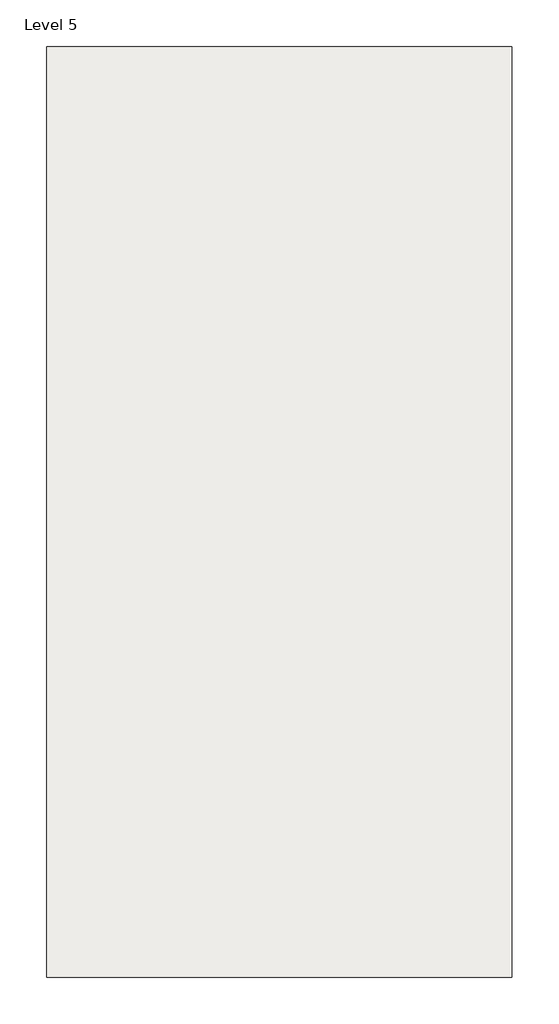
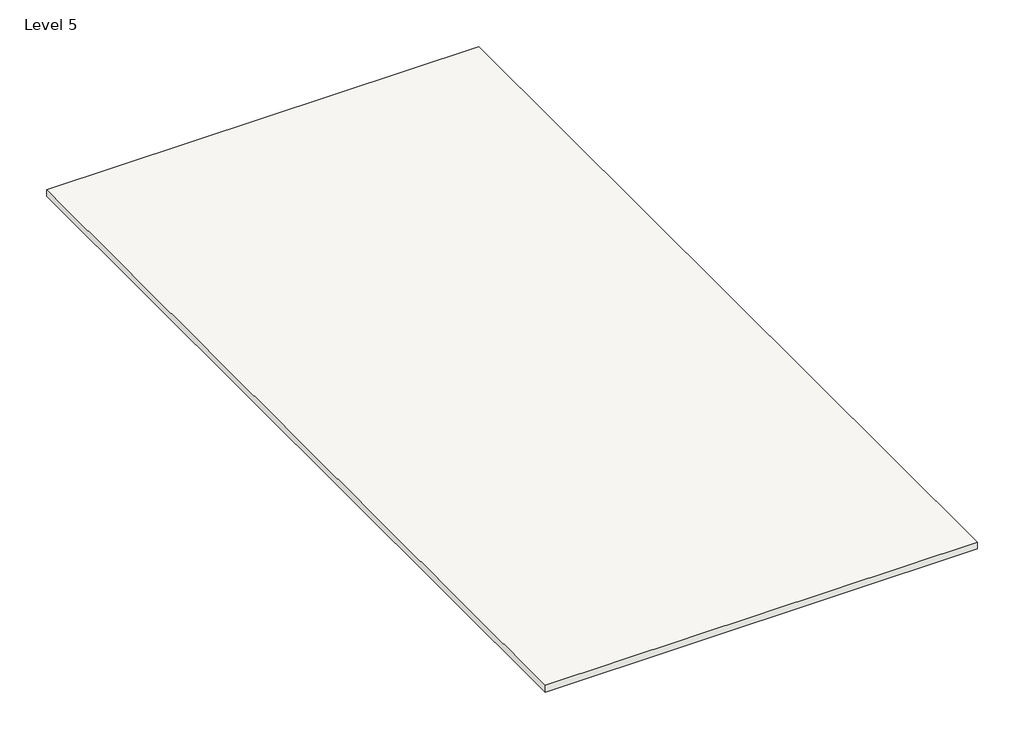
# One storey: 1 roof.
"""IFC4 building model written with IfcOpenShell, lengths in millimetres."""

from ifc_helpers import new_model, si_unit, frame, origin, place, context, project, spatial, polyline, outline, extrude, element, save

model = new_model("IFC4")

# Units and contexts
model_context = context("Model", 3, world=origin())
ifc_project = project(units=[si_unit("LENGTHUNIT", "METRE", prefix="MILLI")], contexts=[model_context])

# Site, building, storey
site = spatial("IfcSite", under=ifc_project)
building = spatial("IfcBuilding", under=site)
storey = spatial("IfcBuildingStorey", under=building, Name="Level 5", Elevation=12192.0)

# Roof
placement = place(None, origin())
element("IfcRoof", 1, ObjectType="Generic - 12\"", at=placement, inside=storey, context=model_context, shape_type="SweptSolid", body=[
    extrude(outline(polyline([(1270.0, 14224.0), (10414.0, 14224.0), (10414.0, -4064.0), (1270.0, -4064.0), (1270.0, 14224.0)])), frame((0.0, 0.0, 12192.0), z_axis=(0.0, 0.0, 1.0), x_axis=(1.0, 0.0, 0.0)), (0.0, 0.0, 1.0), 152.4),
])

save(model, "model.ifc")

# Revit data of these elements
# Type "Generic - 12\""
#   Assembly Code = "B1020"
#   Layers, outside or top first: 0' - 6" "Tile, Porcelain, 4in" (function 1)
# Element 1 (IfcRoof, "Generic - 12\"")
#   built-in parameter 1001705 = 40.5 (stored number, unit not read)
#   built-in parameter 1001710 = 33615
#   Phase Created = New Construction
#   Materials on its faces: "Wood - Stained", "Tile, Porcelain, 4in"
# Materials
#   "Tile, Porcelain, 4in": class "Generic", colour RGB 89 87 158, transparency 0, Description = "Porcelain tile, 4\", white", Cost = 0
#   "Wood - Stained": class "Wood", colour RGB 224 178 126, transparency 0, Cost = 0
